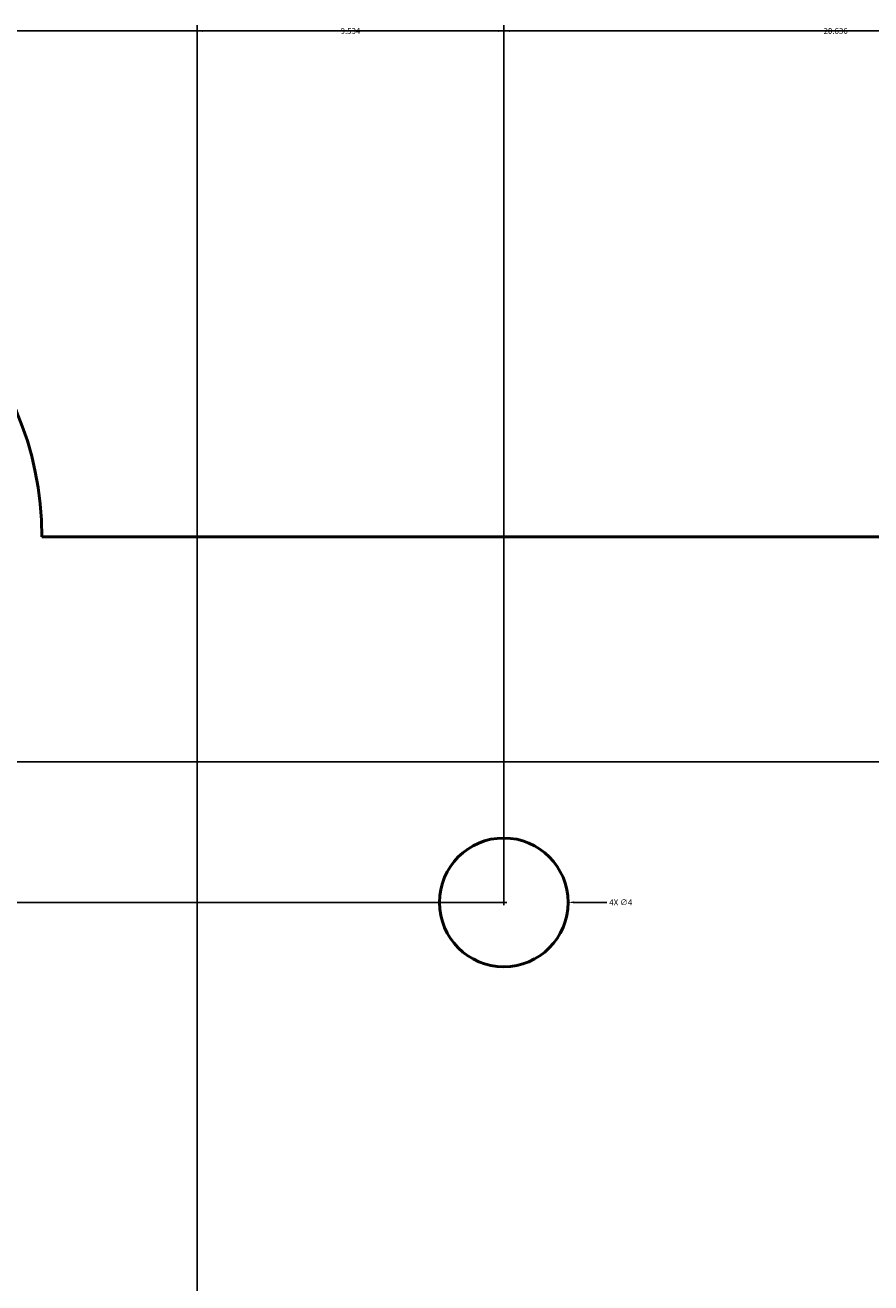
# Model space of a CAD drawing. Units: inches. Extents: x -14 to 108, y -9 to 83.
# Tile 6 of 13: x 12 to 38, y 44 to 83. Entities that reach past the tile are written whole.
import ezdxf

# ---------------------------------------------------------------- set-up
doc = ezdxf.new("R2010")
doc.units = ezdxf.units.IN
doc.header["$MEASUREMENT"] = 0
doc.layers.add('M-DIMS', color=2, linetype='Continuous', lineweight=18)
doc.layers.add('M-OUTL', color=7, linetype='Continuous', lineweight=50)
doc.styles.get("Standard").update_dxf_attribs({"font": 'arial.ttf'})
doc.dimstyles.get("Standard").update_dxf_attribs({"dimtxt": 0.18, "dimasz": 0.18, "dimexe": 0.18, "dimexo": 0.0625, "dimgap": 0.09, "dimtad": 0, "dimtih": 1, "dimtoh": 1, "dimzin": 0, "dimdsep": 46, "dimtxsty": 'Standard', "dimcen": 0.09, "dimadec": 0, "dimazin": 0, "dimtfac": 1, "dimtofl": 0, "dimtmove": 0, "dimatfit": 3, "dimfxl": 1, "dimtolj": 1, "dimtzin": 0, "dimarcsym": 0})

# ---------------------------------------------------------------- blocks, each defined once
blk = doc.blocks.new('HOLE-D4')
blk.add_circle((2, 2), 2)
blk = doc.blocks.new('*D4')
at = {"layer": 'Defpoints', "color": 0, "transparency": 16777216}
for p in [(102.098, 82.834), (-7.902, 67.119), (102.098, 67.119)]:
    blk.add_point(p, dxfattribs=at)
at = {"layer": 'M-DIMS', "color": 0, "lineweight": -2, "transparency": 16777216}
for p, q in [((-7.902, 67.182), (-7.902, 83.014)), ((102.098, 67.182), (102.098, 83.014)), ((-7.722, 82.834), (46.818, 82.834)), ((101.918, 82.834), (47.378, 82.834))]:
    blk.add_line(p, q, dxfattribs=at)
at = {"layer": 'M-DIMS', "color": 0, "transparency": 16777216}
for points in [[(-7.722, 82.864), (-7.722, 82.804), (-7.902, 82.834)], [(101.918, 82.864), (101.918, 82.804), (102.098, 82.834)]]:
    blk.add_solid(points, dxfattribs=at)
at = {"layer": 'M-DIMS', "color": 0, "transparency": 16777216, "insert": (47.098, 82.834), "char_height": 0.18, "attachment_point": 5}
blk.add_mtext('\\A1;110', dxfattribs=at)
blk = doc.blocks.new('*D13')
at = {"layer": 'Defpoints', "color": 0, "transparency": 16777216}
for p in [(26.462, 82.834), (26.462, 55.756), (16.928, 37.119)]:
    blk.add_point(p, dxfattribs=at)
at = {"layer": 'M-DIMS', "color": 0, "lineweight": -2, "transparency": 16777216}
for p, q in [((16.928, 37.182), (16.928, 83.014)), ((26.462, 55.818), (26.462, 83.014)), ((17.108, 82.834), (21.301, 82.834)), ((26.282, 82.834), (22.088, 82.834))]:
    blk.add_line(p, q, dxfattribs=at)
at = {"layer": 'M-DIMS', "color": 0, "transparency": 16777216}
for points in [[(17.108, 82.864), (17.108, 82.804), (16.928, 82.834)], [(26.282, 82.864), (26.282, 82.804), (26.462, 82.834)]]:
    blk.add_solid(points, dxfattribs=at)
at = {"layer": 'M-DIMS', "color": 0, "transparency": 16777216, "insert": (21.695, 82.834), "char_height": 0.18, "attachment_point": 5}
blk.add_mtext('\\A1;9.534', dxfattribs=at)
blk = doc.blocks.new('*D15')
at = {"layer": 'Defpoints', "color": 0, "transparency": 16777216}
for p in [(47.098, 82.834), (47.098, 60.119), (26.462, 55.756)]:
    blk.add_point(p, dxfattribs=at)
at = {"layer": 'M-DIMS', "color": 0, "lineweight": -2, "transparency": 16777216}
for p, q in [((26.462, 55.818), (26.462, 83.014)), ((47.098, 60.182), (47.098, 83.014)), ((26.642, 82.834), (36.315, 82.834)), ((46.918, 82.834), (37.245, 82.834))]:
    blk.add_line(p, q, dxfattribs=at)
at = {"layer": 'M-DIMS', "color": 0, "transparency": 16777216}
for points in [[(26.642, 82.864), (26.642, 82.804), (26.462, 82.834)], [(46.918, 82.864), (46.918, 82.804), (47.098, 82.834)]]:
    blk.add_solid(points, dxfattribs=at)
at = {"layer": 'M-DIMS', "color": 0, "transparency": 16777216, "insert": (36.78, 82.834), "char_height": 0.18, "attachment_point": 5}
blk.add_mtext('\\A1;20.636', dxfattribs=at)
blk = doc.blocks.new('*D18')
at = {"layer": 'Defpoints', "color": 0, "transparency": 16777216}
for p in [(-13.617, 55.756), (26.462, 55.756), (16.928, 37.119)]:
    blk.add_point(p, dxfattribs=at)
at = {"layer": 'M-DIMS', "color": 0, "lineweight": -2, "transparency": 16777216}
for p, q in [((26.399, 55.756), (-13.797, 55.756)), ((-13.617, 55.576), (-13.617, 46.619)), ((-13.617, 37.299), (-13.617, 46.256)), ((16.865, 37.119), (-13.797, 37.119))]:
    blk.add_line(p, q, dxfattribs=at)
at = {"layer": 'M-DIMS', "color": 0, "transparency": 16777216}
for points in [[(-13.647, 55.576), (-13.587, 55.576), (-13.617, 55.756)], [(-13.647, 37.299), (-13.587, 37.299), (-13.617, 37.119)]]:
    blk.add_solid(points, dxfattribs=at)
at = {"layer": 'M-DIMS', "color": 0, "transparency": 16777216, "insert": (-13.617, 46.437), "char_height": 0.18, "attachment_point": 5}
blk.add_mtext('\\A1;18.636', dxfattribs=at)
blk = doc.blocks.new('*D23')
at = {"layer": 'Defpoints', "color": 0, "transparency": 16777216}
for p in [(-13.617, 60.119), (47.098, 60.119), (26.462, 55.756)]:
    blk.add_point(p, dxfattribs=at)
at = {"layer": 'M-DIMS', "color": 0, "lineweight": -2, "transparency": 16777216}
for p, q in [((47.035, 60.119), (-13.797, 60.119)), ((-13.617, 59.939), (-13.617, 58.119)), ((-13.617, 55.936), (-13.617, 57.756)), ((26.399, 55.756), (-13.797, 55.756))]:
    blk.add_line(p, q, dxfattribs=at)
at = {"layer": 'M-DIMS', "color": 0, "transparency": 16777216}
for points in [[(-13.647, 59.939), (-13.587, 59.939), (-13.617, 60.119)], [(-13.647, 55.936), (-13.587, 55.936), (-13.617, 55.756)]]:
    blk.add_solid(points, dxfattribs=at)
at = {"layer": 'M-DIMS', "color": 0, "transparency": 16777216, "insert": (-13.617, 57.937), "char_height": 0.18, "attachment_point": 5}
blk.add_mtext('\\A1;4.364', dxfattribs=at)
blk = doc.blocks.new('*D29')
at = {"layer": 'Defpoints', "color": 0, "transparency": 16777216}
for p in [(24.462, 55.755), (28.462, 55.756)]:
    blk.add_point(p, dxfattribs=at)
at = {"layer": 'M-DIMS', "color": 0, "lineweight": -2, "transparency": 16777216}
for p, q in [((26.372, 55.756), (26.552, 55.756)), ((26.462, 55.666), (26.462, 55.846)), ((29.662, 55.756), (28.642, 55.756))]:
    blk.add_line(p, q, dxfattribs=at)
at = {"layer": 'M-DIMS', "color": 0, "transparency": 16777216}
blk.add_solid([(28.642, 55.786), (28.642, 55.726), (28.462, 55.756)], dxfattribs=at)
at = {"layer": 'M-DIMS', "color": 0, "transparency": 16777216, "insert": (30.1, 55.756), "char_height": 0.18, "attachment_point": 5}
blk.add_mtext('\\A1;4X ∅4', dxfattribs=at)

msp = doc.modelspace()

# ---------------------------------------------------------------- linework, layer by layer
at = {"layer": 'M-OUTL'}
msp.add_lwpolyline([(82.0979, 67.1193), (12.0979, 67.1193)], dxfattribs=at)
msp.add_arc((2.0979, 67.1193), 10, 0, 270, dxfattribs=at)

# ---------------------------------------------------------------- block references
msp.add_blockref('HOLE-D4', (24.4618, 53.7553), dxfattribs=at)

# ---------------------------------------------------------------- dimensions: what is measured, and where the dimension line sits
at = {"layer": 'M-DIMS'}
for base, p1, p2, override, picture, middle in [((102.0979, 82.8343), (-7.9021, 67.1193), (102.0979, 67.1193), {"dimdec": 0, "dimlfac": 1, "dimrnd": 0, "dimzin": 0, "dimdsep": 46, "dimlunit": 2}, '*D4', (47.0979, 82.8343)), ((26.4616, 82.8343), (16.9278, 37.1193), (26.4616, 55.7556), {"dimdec": 3, "dimlfac": 1, "dimrnd": 0, "dimzin": 0, "dimdsep": 46, "dimlunit": 2}, '*D13', (21.6947, 82.8343)), ((47.0979, 82.8343), (26.4616, 55.7556), (47.0979, 60.1193), {"dimdec": 3, "dimlfac": 1, "dimrnd": 0, "dimzin": 0, "dimdsep": 46, "dimlunit": 2}, '*D15', (36.7798, 82.8343))]:
    dim = msp.add_linear_dim(base=base, p1=p1, p2=p2, dimstyle='Standard', override=override, dxfattribs=at)
    dim.commit()
    dim.dimension.update_dxf_attribs({"geometry": picture, "text_midpoint": middle})
for base, p1, p2, picture, middle in [((-13.6171, 60.1193), (26.4616, 55.7556), (47.0979, 60.1193), '*D23', (-13.6171, 57.9375)), ((-13.6171, 55.7556), (16.9278, 37.1193), (26.4616, 55.7556), '*D18', (-13.6171, 46.4375))]:
    dim = msp.add_linear_dim(base=base, p1=p1, p2=p2, angle=90, dimstyle='Standard', override={"dimdec": 3, "dimlfac": 1, "dimrnd": 0, "dimzin": 0, "dimdsep": 46, "dimlunit": 2}, dxfattribs=at)
    dim.commit()
    dim.dimension.update_dxf_attribs({"geometry": picture, "text_midpoint": middle})
dim = msp.add_diameter_dim_2p(p1=(24.4616, 55.7553), p2=(28.4616, 55.756), text='4X <>', dimstyle='Standard', override={"dimdec": 0, "dimlfac": 1, "dimrnd": 0, "dimzin": 0, "dimdsep": 46, "dimlunit": 2}, dxfattribs=at)
dim.commit()
dim.dimension.update_dxf_attribs({"geometry": '*D29', "text_midpoint": (29.6616, 55.7562), "dimtype": 163})

doc.saveas('drawing.dxf')
